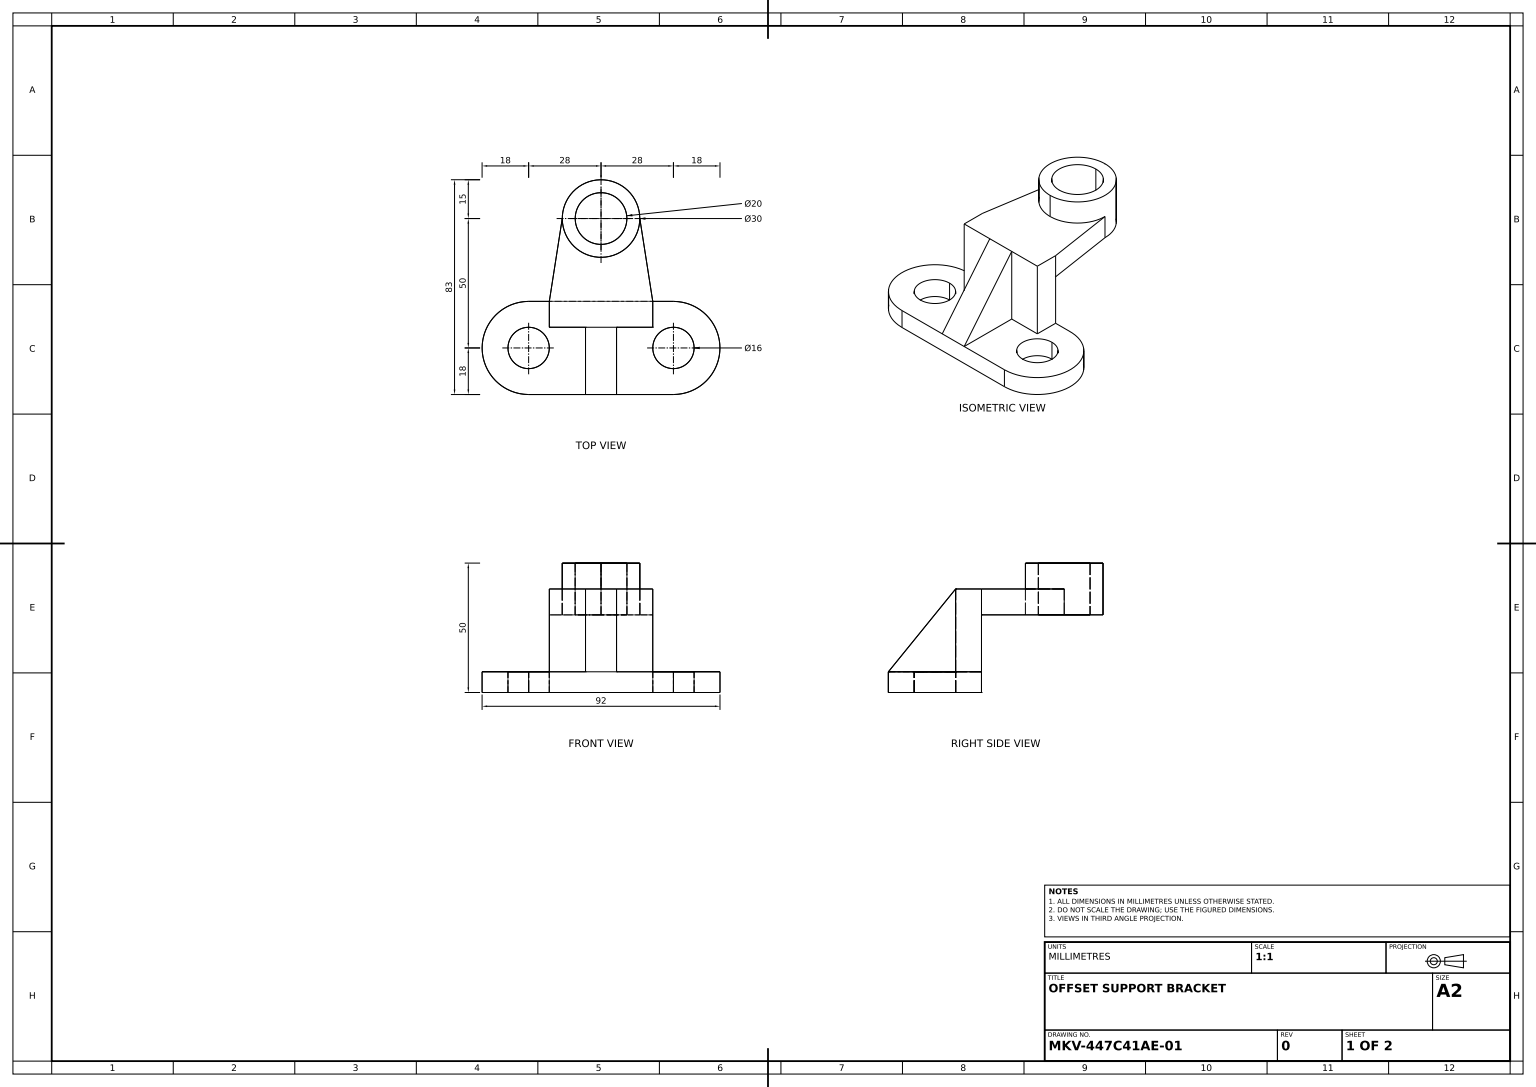
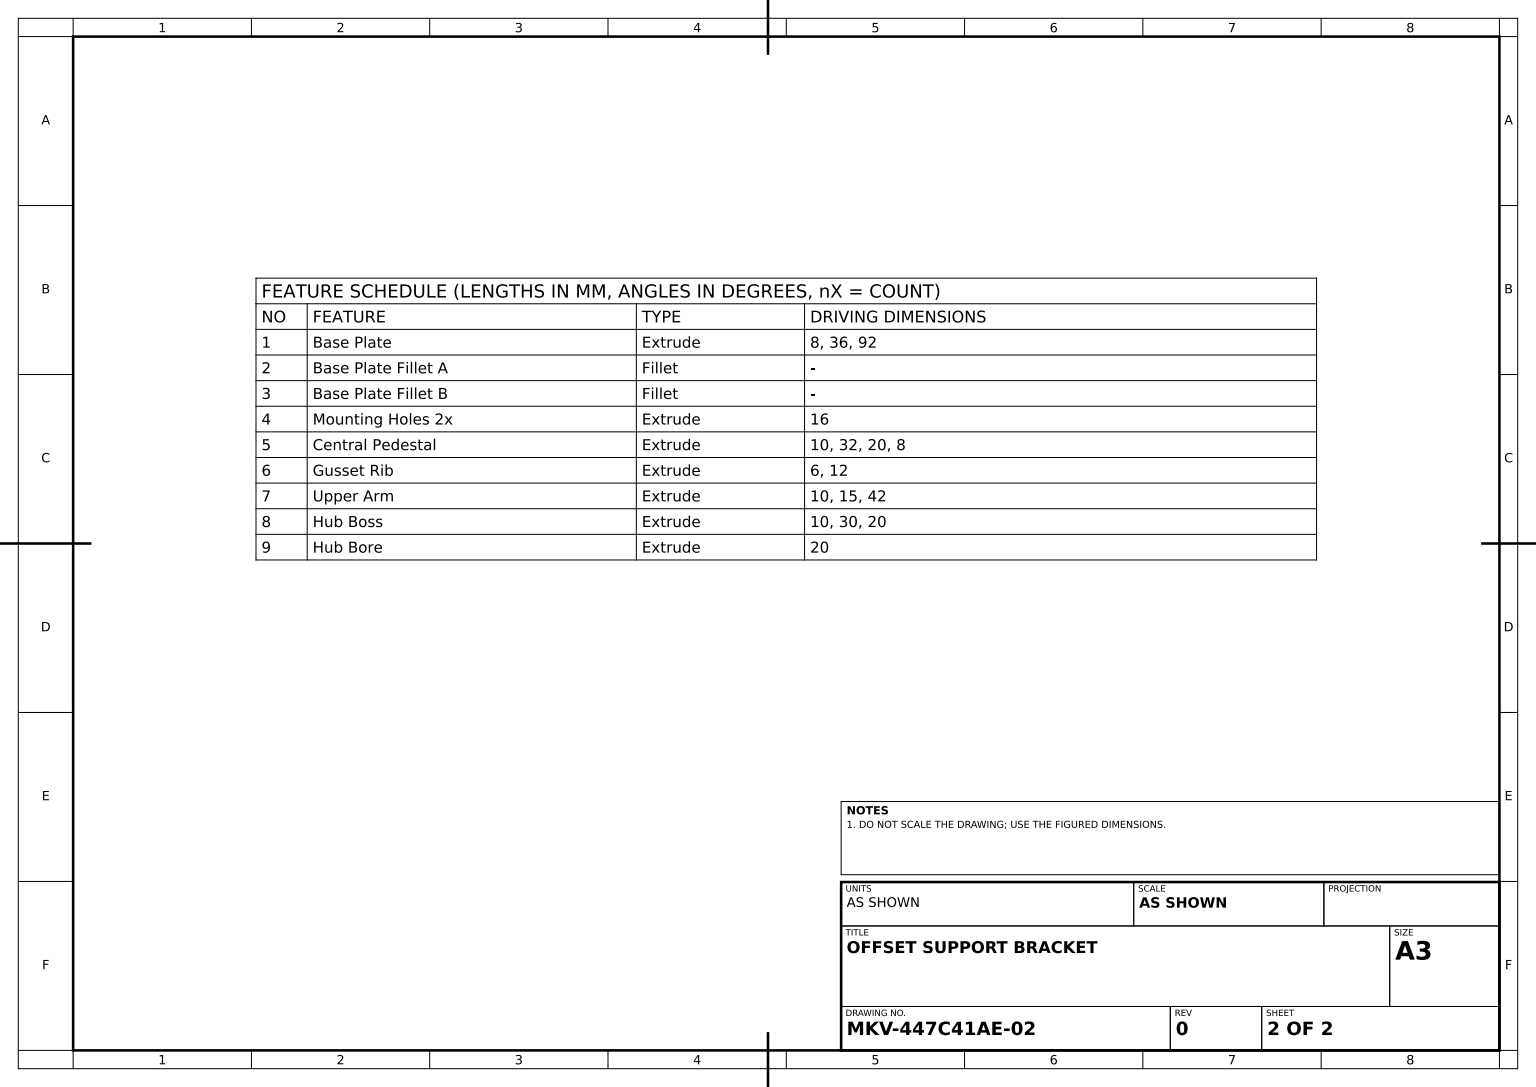
from build123d import *

# Parameters (mm, degrees)
BASE_PLATE_SKETCH_W        = 92
BASE_PLATE_SKETCH_H        = 36
BASE_PLATE_DEPTH           = 8
BASE_PLATE_FILLET_A_RADIUS = 18
BASE_PLATE_FILLET_A_LENGTH = 8
BASE_PLATE_FILLET_B_RADIUS = 18
BASE_PLATE_FILLET_B_LENGTH = 8
MOUNTING_HOLES_SKETCH_R    = 8
MOUNTING_HOLES_2X_DEPTH    = 51.039984013
PEDESTAL_SKETCH_W          = 40
PEDESTAL_SKETCH_H          = 32
CENTRAL_PEDESTAL_DEPTH     = 10
GUSSET_RIB_DEPTH           = 12
UPPER_ARM_DEPTH            = 10
HUB_START                  = 10
HUB_BOSS_SKETCH_R          = 15
HUB_BOSS_SKETCH_R_2        = 10
HUB_BOSS_DEPTH             = 10
HUB_BORE_SKETCH_R          = 10
HUB_BORE_DEPTH             = 90.112288715


with BuildPart() as part:
    # Base Plate Sketch → Base Plate (new body)
    with BuildSketch(Plane(origin=(0, 0, 0), x_dir=(1, 0, 0), z_dir=(0, 1, 0))):
        Rectangle(BASE_PLATE_SKETCH_W, BASE_PLATE_SKETCH_H)
    extrude(amount=BASE_PLATE_DEPTH)

    # Base Plate Fillet A: full round fillet: the end face becomes a half cylinder, R = half its width
    base_plate_fillet_a_face = Plane((46, 4, 0), x_dir=(0, -1, 0), z_dir=(1, 0, 0))  # on the end face: x along it, z out of the body
    base_plate_fillet_a_slab = base_plate_fillet_a_face.offset(-BASE_PLATE_FILLET_A_RADIUS / 2) * Box(BASE_PLATE_FILLET_A_LENGTH, 2 * BASE_PLATE_FILLET_A_RADIUS, BASE_PLATE_FILLET_A_RADIUS, mode=Mode.PRIVATE)  # the body's end, R deep
    base_plate_fillet_a_round = Plane((28, 4, 0), x_dir=(1, 0, 0), z_dir=(0, -1, 0)) * Cylinder(BASE_PLATE_FILLET_A_RADIUS, BASE_PLATE_FILLET_A_LENGTH, mode=Mode.PRIVATE)  # its axis R under the face
    add(base_plate_fillet_a_slab - base_plate_fillet_a_round, mode=Mode.SUBTRACT)

    # Base Plate Fillet B: full round fillet: the end face becomes a half cylinder, R = half its width
    base_plate_fillet_b_face = Plane((-46, 4, 0), x_dir=(0, 1, 0), z_dir=(-1, 0, 0))  # on the end face: x along it, z out of the body
    base_plate_fillet_b_slab = base_plate_fillet_b_face.offset(-BASE_PLATE_FILLET_B_RADIUS / 2) * Box(BASE_PLATE_FILLET_B_LENGTH, 2 * BASE_PLATE_FILLET_B_RADIUS, BASE_PLATE_FILLET_B_RADIUS, mode=Mode.PRIVATE)  # the body's end, R deep
    base_plate_fillet_b_round = Plane((-28, 4, 0), x_dir=(-1, 0, 0), z_dir=(0, 1, 0)) * Cylinder(BASE_PLATE_FILLET_B_RADIUS, BASE_PLATE_FILLET_B_LENGTH, mode=Mode.PRIVATE)  # its axis R under the face
    add(base_plate_fillet_b_slab - base_plate_fillet_b_round, mode=Mode.SUBTRACT)

    # Mounting Holes Sketch → Mounting Holes 2x (cut, through all)
    with BuildSketch(Plane(origin=(0, 8, 0), x_dir=(1, 0, 0), z_dir=(0, 1, 0))):
        with Locations(Location((-28, 0, 0), (0, 0, 270))):
            Circle(MOUNTING_HOLES_SKETCH_R)
        with Locations(Location((28, 0, 0), (0, 0, 270))):
            Circle(MOUNTING_HOLES_SKETCH_R)
    extrude(amount=-MOUNTING_HOLES_2X_DEPTH, mode=Mode.SUBTRACT)

    # Pedestal Sketch → Central Pedestal (add)
    with BuildSketch(Plane(origin=(0, 0, -18), x_dir=(-1, 0, 0), z_dir=(0, 0, -1))):
        with Locations((0, 24)):
            Rectangle(PEDESTAL_SKETCH_W, PEDESTAL_SKETCH_H)
    extrude(amount=-CENTRAL_PEDESTAL_DEPTH)

    # Gusset Rib Sketch → Gusset Rib (add)
    with BuildSketch(Plane(origin=(-6, 0, 0), x_dir=(0, 0, -1), z_dir=(1, 0, 0))):
        Polygon((8, 40), (-18, 8), (8, 8), align=None)
    extrude(amount=GUSSET_RIB_DEPTH)

    # Upper Arm Sketch → Upper Arm (add)
    with BuildSketch(Plane(origin=(0, 40, 0), x_dir=(1, 0, 0), z_dir=(0, 1, 0))):
        with BuildLine():
            Line((-20, 18), (20, 18))
            Line((20, 18), (15, 50))
            ThreePointArc((15, 50), (0, 65), (-15, 50))
            Line((-15, 50), (-20, 18))
        make_face()
    extrude(amount=-UPPER_ARM_DEPTH)

    # Hub Boss Sketch → Hub Boss (add)
    with BuildSketch(Plane(origin=(0, 40, 0), x_dir=(1, 0, 0), z_dir=(0, 1, 0)).offset(HUB_START)):
        with Locations(Location((0, 50, 0), (0, 0, 270))):
            Circle(HUB_BOSS_SKETCH_R)
        with Locations(Location((0, 50, 0), (0, 0, 270))):
            Circle(HUB_BOSS_SKETCH_R_2, mode=Mode.SUBTRACT)
    extrude(amount=-HUB_BOSS_DEPTH)

    # Hub Bore Sketch → Hub Bore (cut, through all)
    with BuildSketch(Plane(origin=(0, 40, 0), x_dir=(1, 0, 0), z_dir=(0, 1, 0))):
        with Locations(Location((0, 50, 0), (0, 0, 270))):
            Circle(HUB_BORE_SKETCH_R)
    extrude(amount=-HUB_BORE_DEPTH, mode=Mode.SUBTRACT)


solid = part.part
